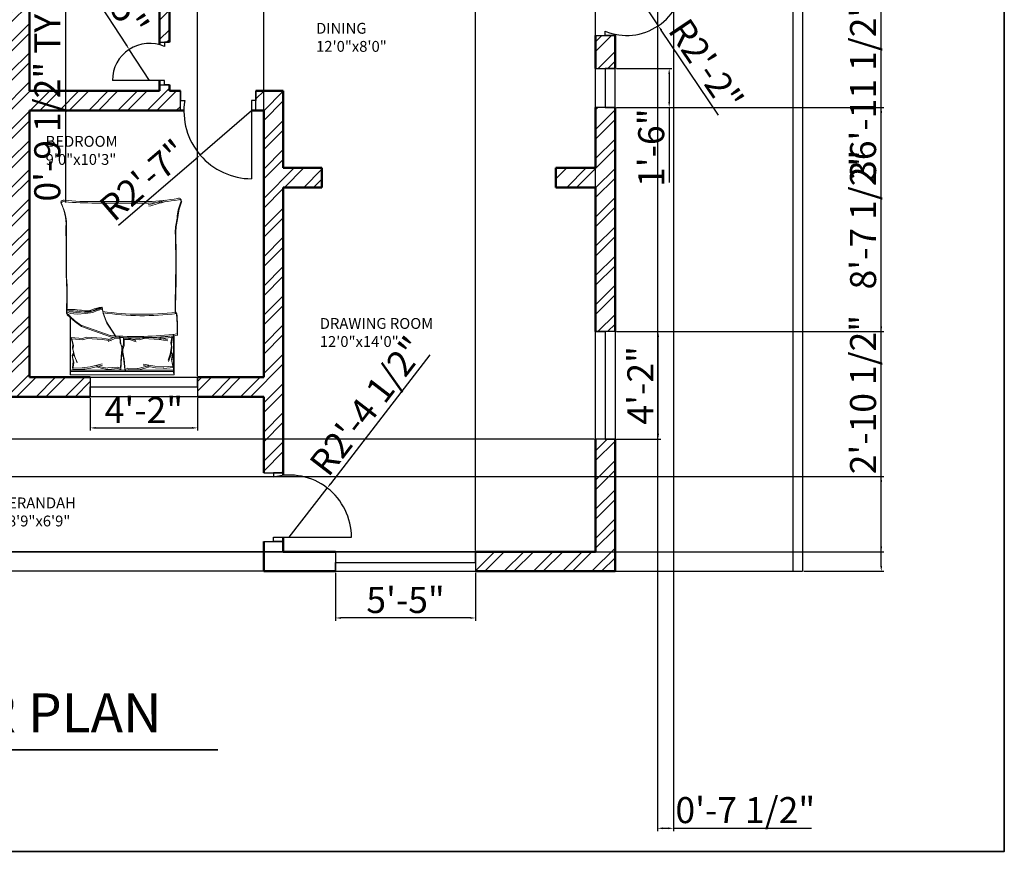
# Model space of a CAD drawing. Units: inches. Extents: x 1990 to 2869, y 1755 to 2533.
# Tile 4 of 6: x 2415 to 2869, y 1755 to 2139. Entities that reach past the tile are written whole.
import ezdxf

# ---------------------------------------------------------------- set-up
doc = ezdxf.new("R2010")
doc.units = ezdxf.units.IN
for name, color, linetype, lineweight in [('A-ANNO-DIMS', 171, 'Continuous', 18), ('A-ANNO-TTLB', 7, 'Continuous', 35), ('A-AREA-IDEN', 7, 'Continuous', 18), ('A-DOOR', 11, 'Continuous', 25), ('A-FLOR', 7, 'Continuous', 25), ('A-FURN', 8, 'Continuous', 18), ('A-GLAZ', 121, 'Continuous', 25), ('A-WALL', 7, 'Continuous', 50), ('A-WALL-SITE', 7, 'Continuous', 30)]:
    doc.layers.add(name, color=color, linetype=linetype, lineweight=lineweight)
doc.layers.add('A-WALL-PATT', color=215, linetype='Continuous', lineweight=13, true_color=0xa953a0)
doc.styles.get("Standard").update_dxf_attribs({"font": 'arial.ttf'})
doc.dimstyles.new('ISO-25', dxfattribs={"dimtxt": 12, "dimasz": 2.5, "dimexe": 1.25, "dimexo": 0.625, "dimtad": 1, "dimdec": 0, "dimlunit": 3, "dimtxsty": 'Standard', "dimcen": 2.5, "dimadec": 0, "dimazin": 0, "dimtfac": 1, "dimtdec": 0, "dimtmove": 0, "dimatfit": 3, "dimfxl": 1, "dimarcsym": 0})

# ---------------------------------------------------------------- blocks, each defined once
blk = doc.blocks.new('*D8')
at = {"layer": 'A-ANNO-DIMS', "color": 0, "lineweight": -2, "transparency": 16777216}
for p, q in [((2447.99, 1964.43), (2447.99, 1949.43)), ((2497.49, 1964.43), (2497.49, 1949.43)), ((2450.49, 1950.68), (2494.99, 1950.68))]:
    blk.add_line(p, q, dxfattribs=at)
at = {"layer": 'A-ANNO-DIMS', "color": 0, "transparency": 16777216}
for points in [[(2450.49, 1951.09), (2450.49, 1950.26), (2447.99, 1950.68)], [(2494.99, 1951.09), (2494.99, 1950.26), (2497.49, 1950.68)]]:
    blk.add_solid(points, dxfattribs=at)
at = {"layer": 'Defpoints', "color": 0, "transparency": 16777216}
for p in [(2447.99, 1965.05), (2497.49, 1965.05), (2497.49, 1950.68)]:
    blk.add_point(p, dxfattribs=at)
at = {"layer": 'A-ANNO-DIMS', "color": 0, "transparency": 16777216, "insert": (2472.74, 1957.33), "char_height": 12, "attachment_point": 5}
blk.add_mtext('4\'-2"', dxfattribs=at)
blk = doc.blocks.new('*D9')
at = {"layer": 'A-ANNO-DIMS', "color": 0, "lineweight": -2, "transparency": 16777216}
for p, q in [((2561.08, 1883.93), (2561.08, 1861.8)), ((2625.68, 1883.93), (2625.68, 1861.8)), ((2623.18, 1863.05), (2563.58, 1863.05))]:
    blk.add_line(p, q, dxfattribs=at)
at = {"layer": 'A-ANNO-DIMS', "color": 0, "transparency": 16777216}
for points in [[(2563.58, 1863.47), (2563.58, 1862.64), (2561.08, 1863.05)], [(2623.18, 1863.47), (2623.18, 1862.64), (2625.68, 1863.05)]]:
    blk.add_solid(points, dxfattribs=at)
at = {"layer": 'Defpoints', "color": 0, "transparency": 16777216}
for p in [(2561.08, 1884.55), (2625.68, 1884.55), (2561.08, 1863.05)]:
    blk.add_point(p, dxfattribs=at)
at = {"layer": 'A-ANNO-DIMS', "color": 0, "transparency": 16777216, "insert": (2593.38, 1869.78), "char_height": 12, "attachment_point": 5}
blk.add_mtext('5\'-5"', dxfattribs=at)
blk = doc.blocks.new('*D10')
at = {"layer": 'A-ANNO-DIMS', "color": 0, "lineweight": -2, "transparency": 16777216}
for p, q in [((2690.6, 1995.05), (2711.1, 1995.05)), ((2709.85, 1948.05), (2709.85, 1992.55)), ((2690.6, 1945.55), (2711.1, 1945.55))]:
    blk.add_line(p, q, dxfattribs=at)
at = {"layer": 'A-ANNO-DIMS', "color": 0, "transparency": 16777216}
for points in [[(2709.44, 1992.55), (2710.27, 1992.55), (2709.85, 1995.05)], [(2709.44, 1948.05), (2710.27, 1948.05), (2709.85, 1945.55)]]:
    blk.add_solid(points, dxfattribs=at)
at = {"layer": 'Defpoints', "color": 0, "transparency": 16777216}
for p in [(2689.97, 1995.05), (2709.85, 1995.05), (2689.97, 1945.55)]:
    blk.add_point(p, dxfattribs=at)
at = {"layer": 'A-ANNO-DIMS', "color": 0, "transparency": 16777216, "insert": (2703.2, 1970.3), "char_height": 12, "attachment_point": 5, "rotation": 90}
blk.add_mtext('4\'-2"', dxfattribs=at)
blk = doc.blocks.new('*D15')
at = {"layer": 'A-ANNO-DIMS', "color": 0, "lineweight": -2, "transparency": 16777216}
for p, q in [((2690.6, 2116.37), (2716.2, 2116.37)), ((2714.95, 2113.87), (2714.95, 2100.87)), ((2690.6, 2098.37), (2716.2, 2098.37)), ((2714.95, 2098.37), (2714.95, 2063.85))]:
    blk.add_line(p, q, dxfattribs=at)
at = {"layer": 'A-ANNO-DIMS', "color": 0, "transparency": 16777216}
for points in [[(2714.53, 2113.87), (2715.37, 2113.87), (2714.95, 2116.37)], [(2714.53, 2100.87), (2715.37, 2100.87), (2714.95, 2098.37)]]:
    blk.add_solid(points, dxfattribs=at)
at = {"layer": 'Defpoints', "color": 0, "transparency": 16777216}
for p in [(2689.97, 2116.37), (2689.97, 2098.37), (2714.95, 2098.37)]:
    blk.add_point(p, dxfattribs=at)
at = {"layer": 'A-ANNO-DIMS', "color": 0, "transparency": 16777216, "insert": (2708.2, 2079.86), "char_height": 12, "attachment_point": 5, "rotation": 90}
blk.add_mtext('1\'-6"', dxfattribs=at)
blk = doc.blocks.new('BED-DOUBLE')
for p, q in [((3.47, 63.33), (3.47, 81.44)), ((3.47, 81.44), (51.49, 81.44)), ((3.47, 79.91), (51.27, 79.91)), ((3.48, 63.33), (3.48, 81.44)), ((3.48, 79.91), (51.27, 79.91)), ((3.7, 62.69), (3.7, 80.8)), ((3.7, 62.69), (3.7, 80.8)), ((3.7, 79.27), (51.49, 79.27)), ((3.7, 79.27), (51.49, 79.27)), ((3.89, 78.13), (4.47, 74.95)), ((3.89, 78.13), (4.47, 74.95)), ((3.9, 78.11), (8.18, 78.43)), ((3.9, 78.11), (8.18, 78.43)), ((4.12, 77.49), (4.7, 74.31)), ((4.12, 77.49), (4.7, 74.31)), ((4.13, 77.47), (8.41, 77.8)), ((4.13, 77.47), (8.41, 77.8)), ((8.18, 78.43), (8.28, 78.42)), ((8.18, 78.43), (8.28, 78.42)), ((8.28, 78.42), (12.11, 78.13)), ((8.28, 78.42), (12.11, 78.13)), ((8.41, 77.8), (8.51, 77.78)), ((8.41, 77.8), (8.51, 77.78)), ((8.51, 77.78), (12.34, 77.49)), ((8.51, 77.78), (12.34, 77.49)), ((12.11, 78.13), (17.6, 77.11)), ((12.11, 78.13), (17.6, 77.11)), ((12.34, 77.49), (17.83, 76.48)), ((12.34, 77.49), (17.83, 76.48)), ((14.85, 77.69), (16.88, 78.42)), ((14.85, 77.69), (16.88, 78.42)), ((15.08, 77.05), (17.11, 77.78)), ((15.08, 77.05), (17.11, 77.78)), ((16.88, 78.42), (19.77, 79.14)), ((16.88, 78.42), (19.77, 79.14)), ((17.11, 77.78), (20, 78.5)), ((17.11, 77.78), (20, 78.5)), ((19.77, 79.14), (20.09, 79.14)), ((19.77, 79.14), (20.09, 79.14)), ((20, 78.5), (20.32, 78.5)), ((20, 78.5), (20.32, 78.5)), ((20.09, 79.14), (24.54, 78.99)), ((20.09, 79.14), (24.54, 78.99)), ((20.32, 78.5), (24.77, 78.36)), ((20.32, 78.5), (24.77, 78.36)), ((24.54, 78.99), (25.98, 79.57)), ((24.54, 78.99), (25.98, 79.57)), ((24.77, 78.36), (26.21, 78.93)), ((24.77, 78.36), (26.21, 78.93)), ((25.98, 79.57), (26.56, 74.22)), ((25.98, 79.57), (26.56, 74.22)), ((26.21, 78.93), (26.79, 73.58)), ((26.21, 78.93), (26.79, 73.58)), ((27.98, 78.95), (27.73, 73.58)), ((27.98, 78.95), (27.73, 73.58)), ((28.21, 78.31), (27.96, 72.94)), ((28.2, 78.31), (27.96, 72.94)), ((29.46, 78.46), (27.98, 78.95)), ((29.46, 78.46), (27.98, 78.95)), ((29.68, 77.82), (28.2, 78.31)), ((29.68, 77.82), (28.21, 78.31)), ((33.88, 78.89), (29.46, 78.46)), ((33.88, 78.89), (29.46, 78.46)), ((34.11, 78.25), (29.68, 77.82)), ((34.11, 78.25), (29.68, 77.82)), ((34.2, 78.91), (33.88, 78.89)), ((34.2, 78.91), (33.88, 78.89)), ((34.43, 78.27), (34.11, 78.25)), ((34.43, 78.27), (34.11, 78.25)), ((37.14, 78.36), (34.2, 78.91)), ((37.13, 78.36), (34.2, 78.91)), ((37.36, 77.73), (34.43, 78.27)), ((37.36, 77.73), (34.43, 78.27)), ((41.91, 78.37), (36.49, 77.02)), ((41.91, 78.37), (36.49, 77.02)), ((42.14, 77.73), (36.72, 76.38)), ((42.14, 77.73), (36.72, 76.38)), ((39.2, 77.77), (37.13, 78.36)), ((39.2, 77.77), (37.14, 78.36)), ((39.43, 77.13), (37.36, 77.73)), ((39.43, 77.13), (37.36, 77.73)), ((45.71, 78.9), (41.91, 78.37)), ((45.71, 78.9), (41.91, 78.37)), ((45.94, 78.26), (42.14, 77.73)), ((45.94, 78.26), (42.14, 77.73)), ((50.11, 78.89), (44.71, 78.98)), ((44.71, 78.98), (45.71, 78.9)), ((50.11, 78.89), (44.71, 78.98)), ((44.71, 78.98), (45.71, 78.9)), ((50.34, 78.25), (44.94, 78.34)), ((44.94, 78.34), (45.94, 78.26)), ((50.34, 78.25), (44.94, 78.34)), ((44.94, 78.34), (45.94, 78.26)), ((50.11, 78.89), (49.73, 75.68)), ((50.11, 78.89), (49.73, 75.68)), ((50.34, 78.25), (49.96, 75.04)), ((50.34, 78.25), (49.96, 75.04)), ((51.27, 81.44), (51.27, 54.83)), ((51.27, 81.44), (51.27, 54.83)), ((51.49, 81.44), (51.49, 80.8)), ((51.49, 80.8), (51.49, 54.19)), ((51.49, 80.8), (51.49, 54.19)), ((4.47, 74.95), (4.04, 72.34)), ((4.47, 74.95), (4.04, 72.34)), ((4.7, 74.31), (4.27, 71.7)), ((4.7, 74.31), (4.27, 71.7)), ((5.05, 72.49), (6.06, 75.24)), ((5.05, 72.49), (6.06, 75.24)), ((5.28, 71.85), (6.29, 74.6)), ((5.28, 71.85), (6.29, 74.6)), ((26.56, 74.22), (27.14, 71.04)), ((26.56, 74.22), (27.14, 71.04)), ((26.79, 73.58), (27.37, 70.4)), ((26.79, 73.58), (27.37, 70.4)), ((27.73, 73.58), (27.35, 70.37)), ((27.73, 73.58), (27.35, 70.37)), ((27.96, 72.94), (27.58, 69.73)), ((27.96, 72.94), (27.58, 69.73)), ((49.31, 73.19), (48.13, 75.86)), ((49.31, 73.19), (48.13, 75.86)), ((49.54, 72.55), (48.36, 75.23)), ((49.54, 72.55), (48.36, 75.23)), ((50.11, 69.61), (49.31, 73.19)), ((50.11, 69.61), (49.31, 73.19)), ((49.73, 75.68), (50.33, 73.1)), ((49.73, 75.68), (50.33, 73.1)), ((50.33, 73.1), (49.81, 72.06)), ((50.33, 73.1), (49.81, 72.06)), ((49.96, 75.04), (50.56, 72.47)), ((49.96, 75.04), (50.56, 72.47)), ((4.04, 72.34), (4.62, 71.33)), ((4.04, 72.34), (4.62, 71.33)), ((4.27, 71.7), (4.85, 70.69)), ((4.27, 71.7), (4.85, 70.69)), ((4.47, 68.87), (5.05, 72.49)), ((4.47, 68.87), (5.05, 72.49)), ((4.76, 67.28), (4.47, 68.87)), ((4.76, 67.28), (4.47, 68.87)), ((4.7, 68.23), (5.28, 71.85)), ((4.7, 68.23), (5.28, 71.85)), ((4.99, 66.64), (4.7, 68.23)), ((4.99, 66.64), (4.7, 68.23)), ((27.14, 69.74), (26.56, 67.86)), ((27.14, 69.74), (26.56, 67.86)), ((27.37, 69.1), (26.79, 67.22)), ((27.37, 69.1), (26.79, 67.22)), ((27.14, 71.04), (27.14, 69.74)), ((27.14, 71.04), (27.14, 69.74)), ((27.35, 70.37), (27.44, 69.07)), ((27.35, 70.37), (27.44, 69.07)), ((27.37, 70.4), (27.37, 69.1)), ((27.37, 70.4), (27.37, 69.1)), ((27.44, 69.07), (28.13, 67.23)), ((27.44, 69.07), (28.13, 67.23)), ((27.58, 69.73), (27.66, 68.43)), ((27.58, 69.73), (27.66, 68.43)), ((27.66, 68.43), (28.36, 66.59)), ((27.66, 68.43), (28.36, 66.59)), ((50.34, 68.98), (49.54, 72.55)), ((50.34, 68.98), (49.54, 72.55)), ((49.92, 68.01), (50.11, 69.61)), ((49.92, 68.01), (50.11, 69.61)), ((50.56, 72.47), (50.04, 71.42)), ((50.56, 72.47), (50.04, 71.42)), ((50.15, 67.37), (50.34, 68.98)), ((50.15, 67.37), (50.34, 68.98)), ((4.18, 64.1), (4.76, 67.28)), ((4.18, 64.1), (4.76, 67.28)), ((9.28, 64.82), (4.18, 64.1)), ((9.28, 64.82), (4.18, 64.1)), ((4.41, 63.46), (4.99, 66.64)), ((4.41, 63.46), (4.99, 66.64)), ((9.51, 64.19), (4.41, 63.46)), ((9.51, 64.19), (4.41, 63.46)), ((6.38, 65.81), (10.41, 65.15)), ((6.38, 65.81), (10.41, 65.15)), ((6.61, 65.18), (10.64, 64.51)), ((6.61, 65.18), (10.64, 64.51)), ((10.41, 65.15), (9.28, 64.82)), ((10.41, 65.15), (9.28, 64.82)), ((10.64, 64.51), (9.51, 64.19)), ((10.64, 64.51), (9.51, 64.19)), ((10.41, 65.15), (17.42, 64.72)), ((10.41, 65.15), (17.42, 64.72)), ((10.64, 64.51), (17.65, 64.08)), ((10.64, 64.51), (17.65, 64.08)), ((17.42, 64.72), (19.38, 65.27)), ((17.42, 64.72), (19.38, 65.27)), ((17.65, 64.08), (19.61, 64.63)), ((17.65, 64.08), (19.61, 64.63)), ((19.38, 65.27), (24.52, 64.87)), ((19.38, 65.27), (24.52, 64.87)), ((19.61, 64.63), (24.74, 64.23)), ((19.61, 64.63), (24.74, 64.23)), ((24.1, 65.18), (20.96, 66.27)), ((24.1, 65.18), (20.96, 66.27)), ((24.33, 64.54), (21.19, 65.63)), ((24.33, 64.54), (21.19, 65.63)), ((26.56, 65.18), (24.1, 65.18)), ((26.56, 65.18), (24.1, 65.18)), ((26.79, 64.54), (24.33, 64.54)), ((26.79, 64.54), (24.33, 64.54)), ((26.56, 67.86), (26.56, 65.18)), ((26.56, 67.86), (26.56, 65.18)), ((26.79, 67.22), (26.79, 64.54)), ((26.79, 67.22), (26.79, 64.54)), ((28.13, 67.23), (28.3, 64.55)), ((28.13, 67.23), (28.3, 64.55)), ((28.3, 64.55), (30.75, 64.7)), ((28.3, 64.55), (30.75, 64.7)), ((28.36, 66.59), (28.53, 63.91)), ((28.36, 66.59), (28.53, 63.91)), ((28.53, 63.91), (30.98, 64.06)), ((28.53, 63.91), (30.98, 64.06)), ((30.26, 64.06), (34.45, 57.57)), ((30.26, 64.06), (34.45, 57.57)), ((30.75, 64.7), (33.82, 65.99)), ((30.75, 64.7), (33.82, 65.99)), ((30.98, 64.06), (34.05, 65.35)), ((30.98, 64.06), (34.05, 65.35)), ((40.64, 61.13), (32.31, 64.06)), ((40.64, 61.13), (32.31, 64.06)), ((32.56, 65.81), (36.6, 65.15)), ((32.56, 65.81), (36.6, 65.15)), ((32.79, 65.18), (36.82, 64.51)), ((32.79, 65.18), (36.82, 64.51)), ((36.6, 65.15), (43.61, 64.72)), ((36.6, 65.15), (43.61, 64.72)), ((36.82, 64.51), (43.83, 64.08)), ((36.82, 64.51), (43.83, 64.08)), ((43.61, 64.72), (45.57, 65.27)), ((43.61, 64.72), (45.57, 65.27)), ((43.83, 64.08), (45.79, 64.63)), ((43.83, 64.08), (45.79, 64.63)), ((45.57, 65.27), (50.7, 64.87)), ((45.57, 65.27), (50.7, 64.87)), ((45.79, 64.63), (50.93, 64.23)), ((45.79, 64.63), (50.93, 64.23)), ((50.7, 64.87), (49.92, 68.01)), ((50.7, 64.87), (49.92, 68.01)), ((50.93, 64.23), (50.15, 67.37)), ((50.93, 64.23), (50.15, 67.37)), ((30.49, 63.42), (34.68, 56.93)), ((30.49, 63.42), (34.68, 56.93)), ((40.87, 60.49), (32.53, 63.42)), ((40.87, 60.49), (32.53, 63.42)), ((46.22, 59.11), (40.64, 61.13)), ((46.22, 59.11), (40.64, 61.13)), ((46.45, 58.48), (40.87, 60.49)), ((46.45, 58.48), (40.87, 60.49)), ((49.16, 56.95), (46.22, 59.11)), ((49.16, 56.95), (46.22, 59.11)), ((34.45, 57.57), (36.15, 53.08)), ((34.45, 57.57), (36.15, 53.08)), ((34.68, 56.93), (36.38, 52.44)), ((34.68, 56.93), (36.38, 52.44)), ((49.39, 56.31), (46.45, 58.48)), ((49.39, 56.31), (46.45, 58.48)), ((52.87, 53.7), (49.16, 56.95)), ((52.87, 53.7), (49.16, 56.95)), ((53.1, 53.06), (49.39, 56.31)), ((53.1, 53.06), (49.39, 56.31)), ((36.15, 53.08), (36.46, 51.07)), ((36.15, 53.08), (36.46, 51.07)), ((36.38, 52.44), (36.69, 50.43)), ((36.38, 52.44), (36.69, 50.43)), ((36.46, 51.07), (38.94, 51.69)), ((36.46, 51.07), (38.94, 51.69)), ((36.69, 50.43), (39.17, 51.05)), ((36.69, 50.43), (39.17, 51.05)), ((38.94, 51.69), (40.95, 52.61)), ((38.94, 51.69), (40.95, 52.61)), ((39.17, 51.05), (41.18, 51.97)), ((39.17, 51.05), (41.18, 51.97)), ((40.95, 52.61), (44.36, 53.08)), ((40.95, 52.61), (44.36, 53.08)), ((41.18, 51.97), (44.59, 52.44)), ((41.18, 51.97), (44.59, 52.44)), ((44.36, 53.08), (48.23, 53.39)), ((44.36, 53.08), (48.23, 53.39)), ((44.59, 52.44), (48.46, 52.75)), ((44.59, 52.44), (48.46, 52.75)), ((48.23, 53.39), (51.33, 53.08)), ((48.23, 53.39), (51.33, 53.08)), ((48.46, 52.75), (51.56, 52.44)), ((48.46, 52.75), (51.56, 52.44)), ((51.33, 53.08), (52.87, 53.7)), ((51.33, 53.08), (52.87, 53.7)), ((51.56, 52.44), (53.1, 53.06)), ((51.56, 52.44), (53.1, 53.06)), ((52.95, 51.95), (52.87, 53.7, 3.87)), ((52.95, 51.95), (52.87, 53.7, 3.87)), ((53.18, 51.31), (53.1, 53.06, 3.87)), ((53.18, 51.31), (53.1, 53.06, 3.87)), ((15.06, 2.2), (39.68, 2.2)), ((15.06, 2.2), (39.68, 2.2)), ((15.29, 1.56), (39.91, 1.56)), ((15.29, 1.56), (39.91, 1.56))]:
    blk.add_line(p, q)
for centre, radius, start, end in [((21.36, -100.61), 164.97, 86.0865, 96.7821), ((21.36, -100.61), 164.97, 86.0865, 96.7821), ((21.59, -101.25), 164.97, 86.0865, 96.7821), ((21.59, -101.25), 164.97, 86.0865, 96.7821), ((85.16, 61.35), 83.31, 178.7218, 185.604), ((85.16, 61.35), 83.31, 178.7218, 185.604), ((85.39, 60.71), 83.31, 178.7218, 185.604), ((85.39, 60.71), 83.31, 178.7218, 185.604), ((17.76, -74.87), 129.02, 81.7845, 96.9006), ((17.76, -74.87), 129.02, 81.7845, 96.9006), ((17.98, -75.51), 129.02, 81.7845, 96.9006), ((17.98, -75.51), 129.02, 81.7845, 96.9006), ((-167.31, 50.27), 170.11, 358.4762, 1.0082), ((-167.31, 50.27), 170.11, 358.4762, 1.0082), ((-167.08, 49.63), 170.11, 358.4762, 1.0082), ((-167.08, 49.63), 170.11, 358.4762, 1.0082), ((36.64, 51), 0.185, 160.2464, 271.1377), ((36.64, 51), 0.185, 160.2464, 271.1377), ((31.15, 79.96), 29.65, 280.6617, 289.8806), ((31.15, 79.96), 29.65, 280.6617, 289.8806), ((36.86, 50.36), 0.185, 160.2464, 271.1377), ((36.86, 50.36), 0.185, 160.2464, 271.1377), ((31.38, 79.32), 29.65, 280.6617, 289.8806), ((31.38, 79.32), 29.65, 280.6617, 289.8806), ((43.74, 46.38), 6.22, 78.6608, 113.7384), ((43.74, 46.38), 6.22, 78.6608, 113.7384), ((43.97, 45.74), 6.22, 78.6608, 113.7384), ((43.97, 45.74), 6.22, 78.6608, 113.7384), ((51.33, 88.1), 36.18, 259.8763, 272.5657), ((51.33, 88.1), 36.18, 259.8763, 272.5657), ((51.56, 87.46), 36.18, 259.8763, 272.5657), ((51.56, 87.46), 36.18, 259.8763, 272.5657), ((182.27, 45.13), 129.5, 176.9791, 183.8365), ((182.27, 45.13), 129.5, 176.9791, 183.8365), ((182.49, 44.49), 129.5, 176.9791, 183.8365), ((182.49, 44.49), 129.5, 176.9791, 183.8365), ((484.82, 30.83), 482.31, 178.2277, 181.7185), ((484.82, 30.83), 482.31, 178.2277, 181.7185), ((485.05, 30.19), 482.31, 178.2277, 181.7185), ((485.05, 30.19), 482.31, 178.2277, 181.7185), ((-4508.74, 13.62), 4561.86, 0.00217, 0.28689), ((-4508.74, 13.62), 4561.86, 0.00217, 0.28689), ((-4508.52, 12.98), 4561.86, 0.00217, 0.28689), ((-4508.52, 12.98), 4561.86, 0.00217, 0.28689), ((-26.9, 16.93), 29.63, 346.0648, 358.9113), ((-26.9, 16.93), 29.63, 346.0648, 358.9113), ((-26.67, 16.29), 29.63, 346.0648, 358.9113), ((-26.67, 16.29), 29.63, 346.0648, 358.9113), ((76.16, 12.78), 23.07, 177.4714, 206.4681), ((76.16, 12.78), 23.07, 177.4714, 206.4681), ((-21.66, 11.17), 23.56, 337.9751, 356.652), ((-21.66, 11.17), 23.56, 337.9751, 356.652), ((-21.43, 10.53), 23.56, 337.9751, 356.652), ((-21.43, 10.53), 23.56, 337.9751, 356.652), ((76.39, 12.14), 23.07, 177.4714, 206.4681), ((76.39, 12.14), 23.07, 177.4714, 206.4681), ((1.09, 1.73), 1.09, 146.1736, 293.4781), ((1.09, 1.73), 1.09, 146.1736, 293.4781), ((1.32, 1.09), 1.09, 146.1736, 293.4781), ((1.32, 1.09), 1.09, 146.1736, 293.4781), ((21.43, -119.39), 121.76, 92.9958, 99.4091), ((21.43, -119.39), 121.76, 92.9958, 99.4091), ((21.66, -120.03), 121.76, 92.9958, 99.4091), ((21.65, -120.03), 121.76, 92.9958, 99.4091), ((-17.22, 105.15), 106.46, 283.3832, 287.7053), ((-17.22, 105.15), 106.46, 283.3832, 287.7053), ((-16.99, 104.52), 106.46, 283.3832, 287.7053), ((-16.99, 104.52), 106.46, 283.3832, 287.7053), ((41.15, -130.83), 133.04, 84.4998, 90.6351), ((41.15, -130.83), 133.04, 84.4998, 90.6351), ((41.38, -131.47), 133.04, 84.4998, 90.6351), ((41.38, -131.47), 133.04, 84.4998, 90.6351), ((54.41, 2.57), 1.1, 242.6588, 356.02), ((54.41, 2.57), 1.1, 242.6588, 356.02), ((54.64, 1.93), 1.1, 242.6588, 356.02), ((54.64, 1.93), 1.1, 242.6588, 356.02)]:
    blk.add_arc(centre, radius, start, end)
blk = doc.blocks.new('WIN-49_5IN')
for p, q in [((0, 9), (0, 0)), ((0, 9), (49.5, 9)), ((49.5, 4.5), (49.5, 9)), ((49.5, 9), (49.5, 0)), ((0, 0), (0, 4.5)), ((0, 4.5), (49.5, 4.5)), ((49.5, 0), (0, 0))]:
    blk.add_line(p, q)
blk = doc.blocks.new('WIN-18IN')
for p, q in [((0, 4.5), (0, 9)), ((0, 9), (0, 0)), ((0, 9), (18, 9)), ((18, 0), (18, 9)), ((18, 9), (18, 4.5)), ((18, 4.5), (0, 4.5)), ((0, 0), (18, 0))]:
    blk.add_line(p, q)
blk = doc.blocks.new('*D23')
at = {"layer": 'A-ANNO-DIMS', "color": 0, "lineweight": -2, "transparency": 16777216}
for p, q in [((2435.03, 2169.19), (2437.82, 2169.19)), ((2436.57, 2166.69), (2436.57, 2161.95)), ((2435.03, 2159.45), (2437.82, 2159.45)), ((2436.57, 2159.45), (2436.57, 2054.59))]:
    blk.add_line(p, q, dxfattribs=at)
at = {"layer": 'A-ANNO-DIMS', "color": 0, "transparency": 16777216}
for points in [[(2436.15, 2166.69), (2436.99, 2166.69), (2436.57, 2169.19)], [(2436.15, 2161.95), (2436.99, 2161.95), (2436.57, 2159.45)]]:
    blk.add_solid(points, dxfattribs=at)
at = {"layer": 'Defpoints', "color": 0, "transparency": 16777216}
for p in [(2434.41, 2169.19), (2434.41, 2159.45), (2436.57, 2159.45)]:
    blk.add_point(p, dxfattribs=at)
at = {"layer": 'A-ANNO-DIMS', "color": 0, "transparency": 16777216, "insert": (2429.74, 2105.77), "char_height": 12, "attachment_point": 5, "rotation": 90}
blk.add_mtext('0\'-9 1/2" TYP.', dxfattribs=at)
blk = doc.blocks.new('*D27')
at = {"layer": 'A-ANNO-DIMS', "color": 0, "lineweight": -2, "transparency": 16777216}
for p, q in [((2625.68, 1894.18), (2625.68, 2365.55)), ((2680.97, 1894.18), (2680.97, 2365.55)), ((2628.18, 2364.3), (2678.47, 2364.3)), ((2680.97, 2364.3), (2745.07, 2364.3))]:
    blk.add_line(p, q, dxfattribs=at)
at = {"layer": 'A-ANNO-DIMS', "color": 0, "transparency": 16777216}
for points in [[(2628.18, 2364.72), (2628.18, 2363.88), (2625.68, 2364.3)], [(2678.47, 2364.72), (2678.47, 2363.88), (2680.97, 2364.3)]]:
    blk.add_solid(points, dxfattribs=at)
at = {"layer": 'Defpoints', "color": 0, "transparency": 16777216}
for p in [(2680.97, 2364.3), (2625.68, 1893.55), (2680.97, 1893.55)]:
    blk.add_point(p, dxfattribs=at)
at = {"layer": 'A-ANNO-DIMS', "color": 0, "transparency": 16777216, "insert": (2714.27, 2371.13), "char_height": 12, "attachment_point": 5}
blk.add_mtext('4\'-7 1/2"', dxfattribs=at)
blk = doc.blocks.new('*D28')
at = {"layer": 'A-ANNO-DIMS', "color": 0, "lineweight": -2, "transparency": 16777216}
for p, q in [((2812.72, 1928.2), (2812.72, 2001.34)), ((2150.6, 1928.2), (2813.97, 1928.2)), ((2812.72, 1896.05), (2812.72, 1925.7)), ((2150.6, 1893.55), (2813.97, 1893.55))]:
    blk.add_line(p, q, dxfattribs=at)
at = {"layer": 'A-ANNO-DIMS', "color": 0, "transparency": 16777216}
for points in [[(2812.3, 1925.7), (2813.14, 1925.7), (2812.72, 1928.2)], [(2812.3, 1896.05), (2813.14, 1896.05), (2812.72, 1893.55)]]:
    blk.add_solid(points, dxfattribs=at)
at = {"layer": 'Defpoints', "color": 0, "transparency": 16777216}
for p in [(2149.97, 1928.2), (2812.72, 1928.2), (2149.97, 1893.55)]:
    blk.add_point(p, dxfattribs=at)
at = {"layer": 'A-ANNO-DIMS', "color": 0, "transparency": 16777216, "insert": (2805.89, 1966.02), "char_height": 12, "attachment_point": 5, "rotation": 90}
blk.add_mtext('2\'-10 1/2"', dxfattribs=at)
blk = doc.blocks.new('*D29')
at = {"layer": 'A-ANNO-DIMS', "color": 0, "lineweight": -2, "transparency": 16777216}
for p, q in [((2680.35, 1945.55), (2016.97, 1945.55)), ((2018.22, 1896.05), (2018.22, 1943.05)), ((2680.35, 1893.55), (2016.97, 1893.55))]:
    blk.add_line(p, q, dxfattribs=at)
at = {"layer": 'A-ANNO-DIMS', "color": 0, "transparency": 16777216}
for points in [[(2017.8, 1943.05), (2018.64, 1943.05), (2018.22, 1945.55)], [(2017.8, 1896.05), (2018.64, 1896.05), (2018.22, 1893.55)]]:
    blk.add_solid(points, dxfattribs=at)
at = {"layer": 'Defpoints', "color": 0, "transparency": 16777216}
for p in [(2018.22, 1945.55), (2680.97, 1945.55), (2680.97, 1893.55)]:
    blk.add_point(p, dxfattribs=at)
at = {"layer": 'A-ANNO-DIMS', "color": 0, "transparency": 16777216, "insert": (2011.6, 1919.55), "char_height": 12, "attachment_point": 5, "rotation": 90}
blk.add_mtext('4\'-4"', dxfattribs=at)
blk = doc.blocks.new('*D30')
at = {"layer": 'A-ANNO-DIMS', "color": 0, "lineweight": -2, "transparency": 16777216}
for p, q in [((2690.6, 2098.37), (2813.97, 2098.37)), ((2812.72, 1997.55), (2812.72, 2095.87)), ((2690.6, 1995.05), (2813.97, 1995.05))]:
    blk.add_line(p, q, dxfattribs=at)
at = {"layer": 'A-ANNO-DIMS', "color": 0, "transparency": 16777216}
for points in [[(2812.3, 2095.87), (2813.14, 2095.87), (2812.72, 2098.37)], [(2812.3, 1997.55), (2813.14, 1997.55), (2812.72, 1995.05)]]:
    blk.add_solid(points, dxfattribs=at)
at = {"layer": 'Defpoints', "color": 0, "transparency": 16777216}
for p in [(2689.97, 2098.37), (2812.72, 2098.37), (2689.97, 1995.05)]:
    blk.add_point(p, dxfattribs=at)
at = {"layer": 'A-ANNO-DIMS', "color": 0, "transparency": 16777216, "insert": (2805.89, 2046.71), "char_height": 12, "attachment_point": 5, "rotation": 90}
blk.add_mtext('8\'-7 1/2"', dxfattribs=at)
blk = doc.blocks.new('*D32')
at = {"layer": 'A-ANNO-DIMS', "color": 0, "lineweight": -2, "transparency": 16777216}
for p, q in [((2497.49, 1974.68), (2497.49, 2365.55)), ((2527.97, 1974.68), (2527.97, 2365.55)), ((2499.99, 2364.3), (2525.47, 2364.3)), ((2527.97, 2364.3), (2591.79, 2364.3))]:
    blk.add_line(p, q, dxfattribs=at)
at = {"layer": 'A-ANNO-DIMS', "color": 0, "transparency": 16777216}
for points in [[(2499.99, 2364.72), (2499.99, 2363.88), (2497.49, 2364.3)], [(2525.47, 2364.72), (2525.47, 2363.88), (2527.97, 2364.3)]]:
    blk.add_solid(points, dxfattribs=at)
at = {"layer": 'Defpoints', "color": 0, "transparency": 16777216}
for p in [(2527.97, 2364.3), (2497.49, 1974.05), (2527.97, 1974.05)]:
    blk.add_point(p, dxfattribs=at)
at = {"layer": 'A-ANNO-DIMS', "color": 0, "transparency": 16777216, "insert": (2561.13, 2371.13), "char_height": 12, "attachment_point": 5}
blk.add_mtext('2\'-6 1/2"', dxfattribs=at)
blk = doc.blocks.new('*D39')
at = {"layer": 'A-ANNO-DIMS', "color": 0, "lineweight": -2, "transparency": 16777216}
for p, q in [((2709.55, 2282.43), (2709.55, 1764.83)), ((2716.97, 2282.43), (2716.97, 1764.83)), ((2712.05, 1766.08), (2714.47, 1766.08)), ((2716.97, 1766.08), (2780.58, 1766.08))]:
    blk.add_line(p, q, dxfattribs=at)
at = {"layer": 'A-ANNO-DIMS', "color": 0, "transparency": 16777216}
for points in [[(2712.05, 1766.49), (2712.05, 1765.66), (2709.55, 1766.08)], [(2714.47, 1766.49), (2714.47, 1765.66), (2716.97, 1766.08)]]:
    blk.add_solid(points, dxfattribs=at)
at = {"layer": 'Defpoints', "color": 0, "transparency": 16777216}
for p in [(2709.55, 2283.05), (2716.97, 2283.05), (2716.97, 1766.08)]:
    blk.add_point(p, dxfattribs=at)
at = {"layer": 'A-ANNO-DIMS', "color": 0, "transparency": 16777216, "insert": (2750.03, 1772.91), "char_height": 12, "attachment_point": 5}
blk.add_mtext('0\'-7 1/2"', dxfattribs=at)
blk = doc.blocks.new('*D49')
at = {"layer": 'A-ANNO-DIMS', "color": 0, "lineweight": -2, "transparency": 16777216}
for p, q in [((2777.1, 2328.05), (2813.97, 2328.05)), ((2812.72, 1887.05), (2812.72, 2325.55)), ((2777.1, 1884.55), (2813.97, 1884.55))]:
    blk.add_line(p, q, dxfattribs=at)
at = {"layer": 'A-ANNO-DIMS', "color": 0, "transparency": 16777216}
for points in [[(2812.3, 2325.55), (2813.14, 2325.55), (2812.72, 2328.05)], [(2812.3, 1887.05), (2813.14, 1887.05), (2812.72, 1884.55)]]:
    blk.add_solid(points, dxfattribs=at)
at = {"layer": 'Defpoints', "color": 0, "transparency": 16777216}
for p in [(2776.47, 2328.05), (2812.72, 2328.05), (2776.47, 1884.55)]:
    blk.add_point(p, dxfattribs=at)
at = {"layer": 'A-ANNO-DIMS', "color": 0, "transparency": 16777216, "insert": (2805.89, 2106.3), "char_height": 12, "attachment_point": 5, "rotation": 90}
blk.add_mtext('36\'-11 1/2"', dxfattribs=at)
blk = doc.blocks.new('*D51')
at = {"layer": 'A-ANNO-DIMS', "color": 0, "lineweight": -2, "transparency": 16777216}
for p, q in [((2695.32, 2157.77), (2709.92, 2136.08)), ((2737.62, 2094.9), (2711.31, 2134))]:
    blk.add_line(p, q, dxfattribs=at)
at = {"layer": 'A-ANNO-DIMS', "color": 0, "transparency": 16777216}
blk.add_solid([(2711.66, 2134.24), (2710.97, 2133.77), (2709.92, 2136.08)], dxfattribs=at)
at = {"layer": 'Defpoints', "color": 0, "transparency": 16777216}
for p in [(2695.32, 2157.77), (2709.92, 2136.08)]:
    blk.add_point(p, dxfattribs=at)
at = {"layer": 'A-ANNO-DIMS', "color": 0, "transparency": 16777216, "insert": (2730.68, 2117.12), "char_height": 12, "attachment_point": 5, "rotation": 303.9296}
blk.add_mtext('R2\'-2"', dxfattribs=at)
blk = doc.blocks.new('*D53')
at = {"layer": 'A-ANNO-DIMS', "color": 0, "lineweight": -2, "transparency": 16777216}
for p, q in [((2604.64, 1984.43), (2558.82, 1924.94)), ((2539.79, 1900.24), (2557.29, 1922.96))]:
    blk.add_line(p, q, dxfattribs=at)
at = {"layer": 'A-ANNO-DIMS', "color": 0, "transparency": 16777216}
blk.add_solid([(2558.49, 1925.19), (2559.15, 1924.68), (2557.29, 1922.96)], dxfattribs=at)
at = {"layer": 'Defpoints', "color": 0, "transparency": 16777216}
for p in [(2557.29, 1922.96), (2539.79, 1900.24)]:
    blk.add_point(p, dxfattribs=at)
at = {"layer": 'A-ANNO-DIMS', "color": 0, "transparency": 16777216, "insert": (2577.08, 1959.84), "char_height": 12, "attachment_point": 5, "rotation": 52.3965}
blk.add_mtext('R2\'-4 1/2"', dxfattribs=at)
blk = doc.blocks.new('*D56')
at = {"layer": 'A-ANNO-DIMS', "color": 0, "lineweight": -2, "transparency": 16777216}
for p, q in [((2522.42, 2096.79), (2498.71, 2076.45)), ((2461.03, 2044.14), (2496.81, 2074.83))]:
    blk.add_line(p, q, dxfattribs=at)
at = {"layer": 'A-ANNO-DIMS', "color": 0, "transparency": 16777216}
blk.add_solid([(2496.54, 2075.14), (2497.08, 2074.51), (2498.71, 2076.45)], dxfattribs=at)
at = {"layer": 'Defpoints', "color": 0, "transparency": 16777216}
for p in [(2522.42, 2096.79), (2498.71, 2076.45)]:
    blk.add_point(p, dxfattribs=at)
at = {"layer": 'A-ANNO-DIMS', "color": 0, "transparency": 16777216, "insert": (2473.65, 2063.72), "char_height": 12, "attachment_point": 5, "rotation": 40.6175}
blk.add_mtext('R2\'-7"', dxfattribs=at)
blk = doc.blocks.new('*D60')
at = {"layer": 'A-ANNO-DIMS', "color": 0, "lineweight": -2, "transparency": 16777216}
for p, q in [((2438.87, 2166.74), (2464.62, 2127.26)), ((2475.32, 2110.84), (2465.98, 2125.16))]:
    blk.add_line(p, q, dxfattribs=at)
at = {"layer": 'A-ANNO-DIMS', "color": 0, "transparency": 16777216}
blk.add_solid([(2464.97, 2127.48), (2464.27, 2127.03), (2465.98, 2125.16)], dxfattribs=at)
at = {"layer": 'Defpoints', "color": 0, "transparency": 16777216}
for p in [(2465.98, 2125.16), (2475.32, 2110.84)]:
    blk.add_point(p, dxfattribs=at)
at = {"layer": 'A-ANNO-DIMS', "color": 0, "transparency": 16777216, "insert": (2456.72, 2151.73), "char_height": 12, "attachment_point": 5, "rotation": 303.1079}
blk.add_mtext('R1\'-5"', dxfattribs=at)

msp = doc.modelspace()

# ---------------------------------------------------------------- hatches: boundary and pattern name
at = {"layer": 'A-WALL-PATT'}
h = msp.add_hatch(dxfattribs=at)
h.set_pattern_fill('ANSI32', color=256)
h.paths.add_polyline_path([(2193.46, 2287.55), (2131.97, 2287.55), (2131.97, 2278.55), (2193.46, 2278.55)])
h.paths.add_polyline_path([(2113.97, 2278.55), (2113.97, 2287.55), (2104.97, 2287.55), (2104.97, 2257.5), (2113.97, 2257.5)])
h.paths.add_polyline_path([(2113.97, 2205), (2104.97, 2205), (2104.97, 2166.55), (2140.97, 2166.55), (2140.97, 2160.48), (2149.97, 2160.48), (2149.97, 2166.55), (2170.14, 2166.55), (2170.14, 2175.55), (2113.97, 2175.55)])
h.paths.add_polyline_path([(2278.97, 2287.55), (2244.47, 2287.55), (2244.47, 2278.55), (2274.47, 2278.55), (2274.47, 2200.55), (2226.47, 2200.55), (2226.47, 2219.37), (2221.97, 2219.37), (2221.97, 2175.55), (2221.97, 2166.55), (2226.47, 2166.55), (2226.47, 2196.05), (2274.47, 2196.05), (2274.47, 2166.55), (2284.01, 2166.55), (2284.01, 2171.05), (2284.01, 2175.55), (2278.97, 2175.55), (2278.97, 2278.55)])
h.paths.add_polyline_path([(2226.47, 2283.05), (2226.47, 2287.55), (2217.66, 2287.55), (2217.66, 2283.05), (2217.66, 2278.55), (2221.97, 2278.55), (2221.97, 2255.21), (2226.47, 2255.21), (2226.47, 2278.55)])
h.paths.add_polyline_path([(2560.97, 2328.05), (2551.97, 2328.05), (2269.97, 2328.05), (2269.97, 2319.05), (2278.97, 2319.05), (2410.97, 2319.05), (2410.97, 2187.05), (2346.47, 2187.05), (2346.47, 2175.55), (2319.77, 2175.55), (2319.77, 2166.55), (2346.47, 2166.55), (2346.47, 2128.22), (2350.97, 2128.22), (2350.97, 2178.05), (2410.97, 2178.05), (2410.97, 2175.55), (2410.97, 2106.05), (2350.97, 2106.05), (2350.97, 2108.72), (2348.72, 2108.72), (2346.47, 2108.72), (2346.47, 2106.05), (2342.3, 2106.05), (2342.3, 2097.05), (2346.47, 2097.05), (2350.97, 2097.05), (2410.97, 2097.05), (2410.97, 1974.05), (2373.73, 1974.05), (2373.73, 1965.05), (2419.97, 1965.05), (2447.99, 1965.05), (2447.99, 1969.55), (2447.99, 1974.05), (2419.97, 1974.05), (2419.97, 2097.05), (2484.47, 2097.05), (2489.55, 2097.05), (2489.55, 2106.05), (2484.47, 2106.05), (2484.47, 2108.84), (2482.22, 2108.84), (2479.97, 2108.84), (2479.97, 2106.05), (2419.97, 2106.05), (2419.97, 2175.55), (2419.97, 2178.05), (2479.97, 2178.05), (2479.97, 2128.49), (2484.47, 2128.49), (2484.47, 2166.55), (2511.88, 2166.55), (2511.88, 2171.05), (2511.88, 2175.55), (2484.47, 2175.55), (2484.47, 2187.05), (2479.97, 2187.05), (2419.97, 2187.05), (2419.97, 2319.05), (2551.97, 2319.05), (2560.97, 2319.05)])
h.paths.add_polyline_path([(2586.47, 2292.05), (2560.97, 2292.05), (2551.97, 2292.05), (2551.97, 2175.55), (2547.37, 2175.55), (2547.37, 2166.55), (2556.47, 2166.55), (2556.47, 2175.55), (2556.47, 2205.05), (2604.47, 2205.05), (2604.47, 2166.55), (2608.97, 2166.55), (2608.97, 2175.55), (2608.97, 2205.05), (2608.97, 2228.1), (2604.47, 2228.1), (2604.47, 2209.55), (2556.47, 2209.55), (2556.47, 2283.05), (2586.47, 2283.05)])
h.paths.add_polyline_path([(2691.55, 2292.05), (2690.86, 2292.05), (2636.82, 2292.05), (2636.82, 2283.05), (2691.55, 2283.05)])
h.paths.add_polyline_path([(2725.97, 2292.05), (2716.97, 2292.05), (2709.55, 2292.05), (2709.55, 2287.55), (2709.55, 2283.05), (2716.97, 2283.05), (2716.97, 2263.68), (2725.97, 2263.68)])
h.paths.add_polyline_path([(2725.97, 2199.18), (2716.97, 2199.18), (2716.97, 2180.05), (2716.97, 2175.55), (2650.43, 2175.55), (2650.43, 2166.55), (2680.97, 2166.55), (2680.97, 2159.77), (2689.97, 2159.77), (2689.97, 2166.55), (2725.97, 2166.55)])
h.paths.add_polyline_path([(2536.97, 2061.55), (2554.82, 2061.55), (2554.82, 2070.55), (2536.97, 2070.55), (2536.97, 2097.05), (2536.97, 2106.05), (2524.42, 2106.05), (2524.42, 2101.55), (2524.42, 2097.05), (2527.97, 2097.05), (2527.97, 1974.05), (2497.49, 1974.05), (2497.49, 1965.05), (2527.97, 1965.05), (2527.97, 1929.96), (2536.97, 1929.96)])
h.paths.add_polyline_path([(2689.97, 1945.55), (2685.47, 1945.55), (2680.97, 1945.55), (2680.97, 1893.55), (2625.68, 1893.55), (2625.68, 1884.55), (2689.97, 1884.55), (2689.97, 1893.55)])
h.paths.add_polyline_path([(2168.89, 2070.55), (2149.97, 2070.55), (2149.97, 2116.52), (2145.47, 2116.52), (2140.97, 2116.52), (2140.97, 1977.7), (2145.47, 1977.7), (2145.47, 1977.63), (2149.97, 1977.55), (2149.97, 2061.55), (2168.89, 2061.55)])
h.paths.add_polyline_path([(2302.97, 2097.05), (2306.2, 2097.05), (2306.2, 2106.05), (2293.97, 2106.05), (2293.97, 2097.05), (2293.97, 2070.55), (2269.93, 2070.55), (2269.93, 2061.55), (2293.97, 2061.55), (2293.97, 1930.78), (2302.97, 1930.78), (2302.97, 1965.05), (2324.23, 1965.05), (2324.23, 1969.55), (2324.23, 1974.05), (2302.97, 1974.05)])
h.paths.add_polyline_path([(2149.97, 1928.2), (2145.47, 1928.2), (2140.97, 1928.2), (2140.97, 1889.05), (2140.97, 1884.55), (2178.84, 1884.55), (2178.84, 1889.05), (2178.84, 1893.55), (2149.97, 1893.55)])
h.paths.add_polyline_path([(2302.97, 1898.24), (2298.47, 1898.24), (2293.97, 1898.24), (2293.97, 1893.55), (2243.34, 1893.55), (2243.34, 1884.55), (2302.97, 1884.55)])
h = msp.add_hatch(dxfattribs=at)
h.set_pattern_fill('ANSI32', color=256)
h.paths.add_polyline_path([(2689.97, 2131.55), (2685.47, 2131.55), (2680.97, 2131.55), (2680.97, 2116.37), (2689.97, 2116.37)])
h.paths.add_polyline_path([(2689.97, 2098.37), (2685.47, 2098.37), (2680.97, 2098.37), (2680.97, 2070.55), (2662.63, 2070.55), (2662.63, 2061.55), (2680.97, 2061.55), (2680.97, 1995.05), (2689.97, 1995.05)])

# ---------------------------------------------------------------- linework, layer by layer
at = {"layer": 'A-ANNO-TTLB'}
msp.add_line((2256.16, 1802.33), (2506.84, 1802.33), dxfattribs=at)
msp.add_lwpolyline([(1989.71, 2378.83), (2869.46, 2378.83), (2869.46, 1755.45), (1989.71, 1755.45)], close=True, dxfattribs=at)
at = {"layer": 'A-DOOR'}
for p, q in [((2680.97, 2131.55), (2689.97, 2131.55)), ((2685.47, 2131.55), (2685.47, 2133.55)), ((2689.97, 2131.55), (2685.47, 2131.55)), ((2479.97, 2128.49), (2484.47, 2128.49)), ((2484.47, 2128.49), (2482.22, 2128.49)), ((2482.22, 2128.49), (2482.22, 2126.49)), ((2482.22, 2110.84), (2458.22, 2110.84)), ((2479.97, 2108.84), (2484.47, 2108.84)), ((2482.22, 2108.84), (2482.22, 2110.84)), ((2484.47, 2108.84), (2482.22, 2108.84)), ((2489.55, 2097.05), (2489.55, 2106.05)), ((2489.55, 2106.05), (2489.55, 2101.55)), ((2524.42, 2097.05), (2524.42, 2106.05)), ((2524.42, 2106.05), (2524.42, 2101.55)), ((2489.55, 2101.55), (2491.55, 2101.55)), ((2524.42, 2101.55), (2522.42, 2101.55)), ((2522.42, 2101.55), (2522.42, 2065.55)), ((2527.97, 1929.96), (2536.97, 1929.96)), ((2536.97, 1929.96), (2532.47, 1929.96)), ((2532.47, 1929.96), (2532.47, 1927.96)), ((2527.97, 1898.24), (2536.97, 1898.24)), ((2532.47, 1898.24), (2532.47, 1900.24)), ((2532.47, 1900.24), (2568.47, 1900.24)), ((2536.97, 1898.24), (2532.47, 1898.24))]:
    msp.add_line(p, q, dxfattribs=at)
for centre, radius, start, end in [((2695.32, 2157.77), 26.15, 247.8615, 0), ((2475.32, 2110.84), 17.1, 66.2159, 180), ((2522.42, 2096.79), 31.24, 171.2355, 270), ((2539.79, 1900.24), 28.68, 360, 104.794)]:
    msp.add_arc(centre, radius, start, end, dxfattribs=at)
at = {"layer": 'A-FLOR'}
msp.add_line((2527.97, 1884.55), (2302.97, 1884.55), dxfattribs=at)
at = {"layer": 'A-GLAZ'}
for p, q in [((2561.08, 1893.55), (2561.08, 1886.27)), ((2625.68, 1893.55), (2561.08, 1893.55)), ((2625.68, 1888.64), (2625.68, 1893.55)), ((2625.68, 1893.55), (2625.68, 1884.55)), ((2561.08, 1884.55), (2561.08, 1888.64)), ((2561.08, 1888.64), (2625.68, 1888.64)), ((2561.08, 1886.27), (2561.08, 1884.55)), ((2561.08, 1884.55), (2625.68, 1884.55))]:
    msp.add_line(p, q, dxfattribs=at)
at = {"layer": 'A-WALL'}
for p, q in [((2419.97, 2106.05), (2419.97, 2175.55)), ((2479.97, 2178.05), (2479.97, 2127.3)), ((2484.47, 2166.55), (2484.47, 2128.49)), ((2680.97, 2131.55), (2680.97, 2116.37)), ((2689.97, 2132.18), (2689.97, 2116.37)), ((2479.97, 2110.84), (2479.97, 2106.05)), ((2484.47, 2108.84), (2484.47, 2106.05)), ((2479.97, 2106.05), (2419.97, 2106.05)), ((2489.55, 2106.05), (2484.47, 2106.05)), ((2536.97, 2106.05), (2524.42, 2106.05)), ((2536.97, 2097.05), (2536.97, 2106.05)), ((2680.97, 2098.37), (2680.97, 2070.55)), ((2689.97, 2098.37), (2689.97, 1995.05)), ((2484.47, 2097.05), (2419.97, 2097.05)), ((2419.97, 2097.05), (2419.97, 1974.05)), ((2491.18, 2097.05), (2484.47, 2097.05)), ((2527.97, 2097.05), (2522.42, 2097.05)), ((2527.97, 2097.05), (2527.97, 1974.05)), ((2536.97, 2097.05), (2536.97, 2070.55)), ((2554.82, 2070.55), (2536.97, 2070.55)), ((2554.82, 2070.55), (2554.82, 2061.55)), ((2680.97, 2070.55), (2662.63, 2070.55)), ((2662.63, 2070.55), (2662.63, 2061.55)), ((2554.82, 2061.55), (2536.97, 2061.55)), ((2536.97, 2061.55), (2536.97, 1928.77)), ((2680.97, 2061.55), (2662.63, 2061.55)), ((2680.97, 2061.55), (2680.97, 1995.05)), ((2447.99, 1974.05), (2419.97, 1974.05)), ((2527.97, 1974.05), (2497.49, 1974.05)), ((2419.97, 1965.05), (2373.73, 1965.05)), ((2447.99, 1965.05), (2419.97, 1965.05)), ((2527.97, 1965.05), (2497.49, 1965.05)), ((2527.97, 1965.05), (2527.97, 1929.96)), ((2680.97, 1945.55), (2680.97, 1893.55)), ((2689.97, 1945.55), (2689.97, 1884.55)), ((2527.97, 1898.24), (2527.97, 1884.55)), ((2536.97, 1900.24), (2536.97, 1893.55)), ((2561.08, 1893.55), (2536.97, 1893.55)), ((2680.97, 1893.55), (2625.68, 1893.55)), ((2689.97, 1884.55), (2689.97, 1893.55)), ((2527.97, 1884.55), (2561.08, 1884.55)), ((2625.68, 1884.55), (2689.97, 1884.55))]:
    msp.add_line(p, q, dxfattribs=at)
at = {"layer": 'A-WALL-SITE'}
for p, q in [((2776.47, 2328.05), (2776.47, 1884.55)), ((2771.97, 2323.55), (2771.97, 1884.55)), ((2689.97, 1884.55), (2776.47, 1884.55))]:
    msp.add_line(p, q, dxfattribs=at)

# ---------------------------------------------------------------- block references
at = {"layer": 'A-FURN', "rotation": 180}
msp.add_blockref('BED-DOUBLE', (2490.16, 2056.56), dxfattribs=at)
at = {"layer": 'A-GLAZ', "extrusion": (0, 0, -1), "zscale": -1, "rotation": 90}
msp.add_blockref('WIN-18IN', (-2680.97, 2098.36), dxfattribs=at)
at = {"layer": 'A-GLAZ', "rotation": 270}
msp.add_blockref('WIN-49_5IN', (2680.97, 1995.05), dxfattribs=at)
at = {"layer": 'A-GLAZ'}
msp.add_blockref('WIN-49_5IN', (2447.99, 1965.05), dxfattribs=at)

# ---------------------------------------------------------------- texts
at = {"layer": 'A-ANNO-TTLB', "insert": (2263.7, 1828.32), "char_height": 18, "attachment_point": 1}
msp.add_mtext_dynamic_manual_height_columns('FIRST FLOOR PLAN', width=651.0909, gutter_width=12.5, heights=[0], dxfattribs=at)
at = {"layer": 'A-AREA-IDEN', "char_height": 5, "attachment_point": 1}
for s, width, insert in [('DINING\\P12\'0"x8\'0"', 102.0825, (2552.14, 2137.41)), ('BEDROOM\\P9\'0"x10\'3"', 145.869, (2427.43, 2085.28)), ('DRAWING ROOM\\P12\'0"x14\'0"', 304.4747, (2553.84, 2001.33)), ('VERANDAH\\P18\'9"x6\'9"', 153.7874, (2406.24, 1918.59))]:
    msp.add_mtext_dynamic_manual_height_columns(s, width=width, gutter_width=12.5, heights=[0], dxfattribs=dict(at, insert=insert))

# ---------------------------------------------------------------- dimensions: what is measured, and where the dimension line sits
at = {"layer": 'A-ANNO-DIMS'}
for base, p1, p2, override, picture, middle in [((2527.97, 2364.3), (2497.49, 1974.05), (2527.97, 1974.05), {"dimdec": 1, "dimlfac": 1, "dimrnd": 0, "dimzin": 1, "dimdsep": 46, "dimlunit": 4, "dimfrac": 2}, '*D32', (2561.13, 2371.13)), ((2680.97, 2364.3), (2625.68, 1893.55), (2680.97, 1893.55), {"dimdec": 1, "dimlfac": 1, "dimrnd": 0, "dimzin": 1, "dimdsep": 46, "dimlunit": 4, "dimfrac": 2}, '*D27', (2714.27, 2371.13)), ((2716.97, 1766.08), (2709.55, 2283.05), (2716.97, 2283.05), {"dimdec": 1, "dimlfac": 1, "dimrnd": 0, "dimzin": 1, "dimdsep": 46, "dimlunit": 4, "dimfrac": 2}, '*D39', (2750.03, 1772.91)), ((2497.48914993, 1950.67555943), (2447.98914993, 1965.05122255), (2497.48914993, 1965.05122255), {"dimclrd": 0, "dimclre": 0, "dimclrt": 0}, '*D8', (2472.73914993, 1957.32511605)), ((2561.08, 1863.05), (2625.68, 1884.55), (2561.08, 1884.55), {"dimclrd": 0, "dimclre": 0, "dimclrt": 0}, '*D9', (2593.38, 1869.78))]:
    dim = msp.add_linear_dim(base=base, p1=p1, p2=p2, dimstyle='ISO-25', override=override, dxfattribs=at)
    dim.commit()
    dim.dimension.update_dxf_attribs({"geometry": picture, "text_midpoint": middle})
for base, p1, p2, override, picture, middle in [((2812.72, 2328.05), (2776.47, 1884.55), (2776.47, 2328.05), {"dimdec": 1, "dimlfac": 1, "dimrnd": 0, "dimzin": 1, "dimdsep": 46, "dimlunit": 4, "dimfrac": 2}, '*D49', (2805.89, 2106.3)), ((2714.95, 2098.37), (2689.97, 2116.37), (2689.97, 2098.37), {"dimclrd": 0, "dimclre": 0, "dimclrt": 0}, '*D15', (2708.2, 2079.86)), ((2812.72, 2098.37), (2689.97, 1995.05), (2689.97, 2098.37), {"dimdec": 1, "dimlfac": 1, "dimrnd": 0, "dimzin": 1, "dimdsep": 46, "dimlunit": 4, "dimfrac": 2}, '*D30', (2805.89, 2046.71)), ((2812.7213, 1928.2046), (2149.9713, 1893.5512), (2149.9713, 1928.2046), {"dimdec": 1, "dimlfac": 1, "dimrnd": 0, "dimzin": 1, "dimdsep": 46, "dimlunit": 4, "dimfrac": 2}, '*D28', (2805.8917, 1966.024)), ((2709.85349098, 1995.04794809), (2689.97134122, 1945.54794809), (2689.97134122, 1995.04794809), {"dimclrd": 0, "dimclre": 0, "dimclrt": 0}, '*D10', (2703.20393436, 1970.29794809)), ((2018.22, 1945.55), (2680.97, 1893.55), (2680.97, 1945.55), {"dimdec": 1, "dimlfac": 1, "dimrnd": 0, "dimzin": 1, "dimdsep": 46, "dimlunit": 4, "dimfrac": 2}, '*D29', (2011.6, 1919.55))]:
    dim = msp.add_linear_dim(base=base, p1=p1, p2=p2, angle=90, dimstyle='ISO-25', override=override, dxfattribs=at)
    dim.commit()
    dim.dimension.update_dxf_attribs({"geometry": picture, "text_midpoint": middle})
for center, mpoint, picture, middle in [((2475.32, 2110.84), (2465.98, 2125.16), '*D60', (2456.72, 2151.73)), ((2695.32, 2157.77), (2709.92, 2136.08), '*D51', (2730.68, 2117.12)), ((2522.42, 2096.79), (2498.71, 2076.45), '*D56', (2473.65, 2063.72)), ((2539.79, 1900.24), (2557.29, 1922.96), '*D53', (2577.08, 1959.84))]:
    dim = msp.add_radius_dim(center=center, mpoint=mpoint, dimstyle='ISO-25', override={"dimdec": 1, "dimlfac": 1, "dimrnd": 0, "dimzin": 1, "dimdsep": 46, "dimlunit": 4, "dimfrac": 2}, dxfattribs=at)
    dim.commit()
    dim.dimension.update_dxf_attribs({"geometry": picture, "text_midpoint": middle})
dim = msp.add_linear_dim(base=(2436.57, 2159.45), p1=(2434.41, 2169.19), p2=(2434.41, 2159.45), angle=270, text='<> TYP.', dimstyle='ISO-25', override={"dimdec": 1, "dimlfac": 1, "dimrnd": 0, "dimzin": 1, "dimdsep": 46, "dimlunit": 4, "dimfrac": 2}, dxfattribs=at)
dim.commit()
dim.dimension.update_dxf_attribs({"geometry": '*D23', "text_midpoint": (2429.74, 2105.77)})

doc.saveas('drawing.dxf')
